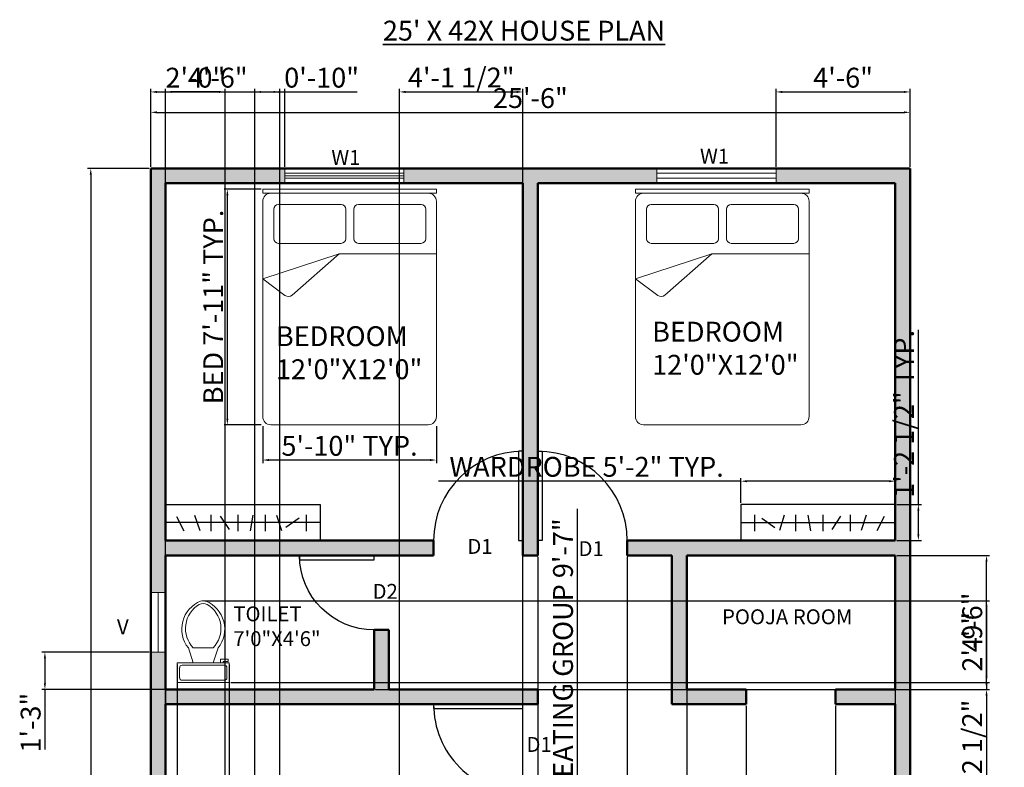
# Model space of a CAD drawing. Units: inches. Extents: x 3655 to 4051, y 2160 to 2854.
# Tile 3 of 3: x 3655 to 4051, y 2552 to 2854. Entities that reach past the tile are written whole.
import ezdxf

# ---------------------------------------------------------------- set-up
doc = ezdxf.new("R2010")
doc.units = ezdxf.units.IN
for name, color, linetype, lineweight in [('A-ANNO-DIMS', 2, 'Continuous', 18), ('A-ANNO-TEXT', 7, 'Continuous', 18), ('A-ANNO-TTLB', 7, 'Continuous', 35), ('A-AREA-IDEN', 7, 'Continuous', 25), ('A-DOOR', 3, 'Continuous', 25), ('A-FLOR-CASE', 8, 'Continuous', 25), ('A-FLOR-FIXT', 9, 'Continuous', 18), ('A-FURN', 8, 'Continuous', 18), ('A-GLAZ', 4, 'Continuous', 18), ('A-WALL', 7, 'Continuous', 50)]:
    doc.layers.add(name, color=color, linetype=linetype, lineweight=lineweight)
doc.layers.add('A-WALL-PATT', color=244, linetype='Continuous', lineweight=13, true_color=0x991b1e)
doc.styles.get("Standard").update_dxf_attribs({"font": 'arial.ttf'})
doc.dimstyles.new('ISO-25', dxfattribs={"dimtxt": 8, "dimasz": 2.5, "dimexe": 1.25, "dimexo": 0.625, "dimtad": 1, "dimdec": 1, "dimlunit": 3, "dimtxsty": 'Standard', "dimcen": 2.5, "dimadec": 0, "dimazin": 0, "dimtfac": 1, "dimtdec": 1, "dimtmove": 0, "dimatfit": 3, "dimfxl": 1, "dimarcsym": 0})

# ---------------------------------------------------------------- blocks, each defined once
blk = doc.blocks.new('*U2')
for p, q in [((0, 0), (0, -6)), ((36, 0), (36, -6))]:
    blk.add_line(p, q)
blk.add_lwpolyline([(0, 0), (0, 36), (1.75, 36), (1.75, 0)], close=True)
blk.add_arc((0, 0), 36, 0, 90)
blk = doc.blocks.new('*U3')
for p, q in [((0, 0), (0, -6)), ((-36, 0), (-36, -6))]:
    blk.add_line(p, q)
blk.add_lwpolyline([(0, 0), (0, 36), (-1.75, 36), (-1.75, 0)], close=True)
blk.add_arc((0, 0), 36, 90, 180)
blk = doc.blocks.new('*U4')
for p, q in [((0, 0), (0, 6)), ((36, 0), (36, 6))]:
    blk.add_line(p, q)
blk.add_lwpolyline([(0, 0), (0, -36), (1.75, -36), (1.75, 0)], close=True)
blk.add_arc((0, 0), 36, 270, 0)
blk = doc.blocks.new('*U5')
for p, q in [((-30, 0), (-30, 6)), ((0, 0), (0, 6))]:
    blk.add_line(p, q)
blk.add_lwpolyline([(0, 0), (0, -30), (-1.75, -30), (-1.75, 0)], close=True)
blk.add_arc((0, 0), 30, 180, 270)
blk = doc.blocks.new('A$C164346CA')
for p, q in [((0, 2.035), (0, 2)), ((1.5, 2.035), (0, 2.035)), ((1.5, 2), (0, 2)), ((1.5, 2), (1.5, 2.035)), ((0, 1.93), (0, 0.07)), ((0.6731, 1.9024), (0.1319, 1.9024)), ((1.364, 1.9024), (0.8228, 1.9024)), ((1.5, 0.07), (1.5, 1.93)), ((0.0919, 1.8624), (0.0919, 1.6069)), ((0.7131, 1.6069), (0.7131, 1.8624)), ((0.7828, 1.8624), (0.7828, 1.6069)), ((1.404, 1.6069), (1.404, 1.8624)), ((0.1319, 1.5669), (0.6731, 1.5669)), ((0.8228, 1.5669), (1.364, 1.5669)), ((0.8395, 1.4761), (0, 1.4761)), ((0.8395, 1.4761), (1.2448, 1.12)), ((1.5, 1.2611), (0.8395, 1.4761)), ((1.3077, 1.1175), (1.5, 1.2611)), ((0.07, 0), (1.43, 0))]:
    blk.add_line(p, q)
for centre, radius, start, end in [((0.07, 1.93), 0.07, 90, 180), ((1.43, 1.93), 0.07, 0, 90), ((0.1319, 1.8624), 0.04, 90, 180), ((0.6731, 1.8624), 0.04, 0, 90), ((0.8228, 1.8624), 0.04, 90, 180), ((1.364, 1.8624), 0.04, 0, 90), ((0.1319, 1.6069), 0.04, 180, 270), ((0.6731, 1.6069), 0.04, 270, 0), ((0.8228, 1.6069), 0.04, 180, 270), ((1.364, 1.6069), 0.04, 270, 0), ((1.2778, 1.1575), 0.05, 228.69584, 306.75789), ((0.07, 0.07), 0.07, 180, 270), ((1.43, 0.07), 0.07, 270, 0)]:
    blk.add_arc(centre, radius, start, end)
blk = doc.blocks.new('*U11')
for p, q in [((9.5, -6), (9.5, -2)), ((-10, -8.5), (-8, -8.5)), ((-10, -9.5), (-10, -8.5)), ((-7, -9.5), (-10, -9.5)), ((-8, -8.5), (-8, -8)), ((-7, -8), (-7, -9.5)), ((-4, -8), (-6, -14)), ((4, -8), (6, -14)), ((4, -14), (-4, -14))]:
    blk.add_line(p, q)
blk.add_lwpolyline([(10.5, -8), (10.5, 0), (-10.5, 0), (-10.5, -8)], close=True)
for points in [[(-9.5, -2), (-9.5, -6)], [(8.5, -1), (-8.5, -1)], [(-8.5, -7), (8.5, -7)]]:
    blk.add_lwpolyline(points)
for centre, radius, start, end in [((-8.62, -1.88), 0.884, 81.8699, 188.1301), ((8.62, -1.88), 0.884, 351.8699, 98.1301), ((-8.62, -6.12), 0.884, 171.8699, 278.1301), ((8.62, -6.12), 0.884, 261.8699, 8.1301), ((3.52, -21.58), 12.17, 141.4691, 247.9714), ((4.2, -21.82), 11.33, 136.3677, 238.9468), ((-3.52, -21.58), 12.17, 292.0284, 38.5307), ((-4.2, -21.82), 11.33, 301.053, 43.6321), ((0, -27.88), 4, 245.7318, 294.2682), ((0, -29), 4, 254.8605, 285.1395)]:
    blk.add_arc(centre, radius, start, end)
blk = doc.blocks.new('*D12')
at = {"layer": 'A-ANNO-DIMS', "color": 0, "lineweight": -2, "transparency": 16777216}
for p, q in [((3707.41, 2794.32), (3707.41, 2817.52)), ((4013.41, 2794.32), (4013.41, 2817.52)), ((3709.91, 2816.27), (4010.91, 2816.27))]:
    blk.add_line(p, q, dxfattribs=at)
at = {"layer": 'A-ANNO-DIMS', "color": 0, "transparency": 16777216}
for points in [[(3709.91, 2816.68), (3709.91, 2815.85), (3707.41, 2816.27)], [(4010.91, 2816.68), (4010.91, 2815.85), (4013.41, 2816.27)]]:
    blk.add_solid(points, dxfattribs=at)
at = {"layer": 'Defpoints', "color": 0, "transparency": 16777216}
for p in [(4013.41, 2816.27), (3707.41, 2793.69), (4013.41, 2793.69)]:
    blk.add_point(p, dxfattribs=at)
at = {"layer": 'A-ANNO-DIMS', "color": 0, "transparency": 16777216, "insert": (3860.41, 2820.98), "char_height": 8, "attachment_point": 5}
blk.add_mtext('25\'-6"', dxfattribs=at)
blk = doc.blocks.new('*D13')
at = {"layer": 'A-ANNO-DIMS', "color": 0, "lineweight": -2, "transparency": 16777216}
for p, q in [((3706.78, 2793.69), (3682, 2793.69)), ((3683.25, 2791.19), (3683.25, 2270.19)), ((3706.78, 2267.69), (3682, 2267.69))]:
    blk.add_line(p, q, dxfattribs=at)
at = {"layer": 'A-ANNO-DIMS', "color": 0, "transparency": 16777216}
for points in [[(3682.83, 2791.19), (3683.66, 2791.19), (3683.25, 2793.69)], [(3682.83, 2270.19), (3683.66, 2270.19), (3683.25, 2267.69)]]:
    blk.add_solid(points, dxfattribs=at)
at = {"layer": 'Defpoints', "color": 0, "transparency": 16777216}
for p in [(3707.41, 2793.69), (3683.25, 2267.69), (3707.41, 2267.69)]:
    blk.add_point(p, dxfattribs=at)
at = {"layer": 'A-ANNO-DIMS', "color": 0, "transparency": 16777216, "insert": (3678.53, 2530.69), "char_height": 8, "attachment_point": 5, "rotation": 90}
blk.add_mtext('43\'-10"', dxfattribs=at)
blk = doc.blocks.new('WARDROBE-RAIL')
for p, q in [((0, 14.59), (62.23, 14.59)), ((62.23, 14.59), (62.23, 0)), ((4.45, 9.69), (7.39, 3.9)), ((11.7, 10.18), (13.76, 4.03)), ((18.16, 10.34), (18.16, 3.85)), ((21.98, 9.84), (25.56, 4.42)), ((29.16, 10.34), (29.16, 3.85)), ((35.17, 10.28), (34.07, 3.88)), ((40.15, 10.34), (40.15, 3.85)), ((44.73, 10.2), (46.68, 4.01)), ((53.78, 8.99), (48.5, 5.2)), ((56.64, 10.34), (56.64, 3.85)), ((62.23, 7.29), (0, 7.29))]:
    blk.add_line(p, q)
blk = doc.blocks.new('WIN-W1-48IN')
for p, q in [((0, 0), (0, 6)), ((48, 4), (0, 4)), ((48, 0), (48, 6)), ((48, 2), (0, 2))]:
    blk.add_line(p, q)
blk = doc.blocks.new('*D16')
at = {"layer": 'A-ANNO-DIMS', "color": 0, "lineweight": -2, "transparency": 16777216}
for p, q in [((3751.9, 2785.3), (3737.04, 2785.3)), ((3738.29, 2692.87), (3738.29, 2782.8)), ((3751.9, 2690.37), (3737.04, 2690.37))]:
    blk.add_line(p, q, dxfattribs=at)
at = {"layer": 'A-ANNO-DIMS', "color": 0, "transparency": 16777216}
for points in [[(3737.87, 2782.8), (3738.71, 2782.8), (3738.29, 2785.3)], [(3737.87, 2692.87), (3738.71, 2692.87), (3738.29, 2690.37)]]:
    blk.add_solid(points, dxfattribs=at)
at = {"layer": 'Defpoints', "color": 0, "transparency": 16777216}
for p in [(3738.29, 2785.3), (3752.53, 2785.3), (3752.53, 2690.37)]:
    blk.add_point(p, dxfattribs=at)
at = {"layer": 'A-ANNO-DIMS', "color": 0, "transparency": 16777216, "insert": (3733.64, 2737.84), "char_height": 8, "attachment_point": 5, "rotation": 90}
blk.add_mtext('BED 7\'-11" TYP.', dxfattribs=at)
blk = doc.blocks.new('*D17')
at = {"layer": 'A-ANNO-DIMS', "color": 0, "lineweight": -2, "transparency": 16777216}
for p, q in [((3752.53, 2689.74), (3752.53, 2674.88)), ((3822.51, 2689.74), (3822.51, 2674.88)), ((3820.01, 2676.13), (3755.03, 2676.13))]:
    blk.add_line(p, q, dxfattribs=at)
at = {"layer": 'A-ANNO-DIMS', "color": 0, "transparency": 16777216}
for points in [[(3755.03, 2676.54), (3755.03, 2675.71), (3752.53, 2676.13)], [(3820.01, 2676.54), (3820.01, 2675.71), (3822.51, 2676.13)]]:
    blk.add_solid(points, dxfattribs=at)
at = {"layer": 'Defpoints', "color": 0, "transparency": 16777216}
for p in [(3752.53, 2690.37), (3822.51, 2690.37), (3752.53, 2676.13)]:
    blk.add_point(p, dxfattribs=at)
at = {"layer": 'A-ANNO-DIMS', "color": 0, "transparency": 16777216, "insert": (3787.52, 2680.84), "char_height": 8, "attachment_point": 5}
blk.add_mtext('5\'-10" TYP.', dxfattribs=at)
blk = doc.blocks.new('*D18')
at = {"layer": 'A-ANNO-DIMS', "color": 0, "lineweight": -2, "transparency": 16777216}
for p, q in [((3945.18, 2667.61), (3823.42, 2667.61)), ((3945.18, 2658.9), (3945.18, 2668.86)), ((4004.91, 2667.61), (3947.68, 2667.61)), ((4007.41, 2658.9), (4007.41, 2668.86))]:
    blk.add_line(p, q, dxfattribs=at)
at = {"layer": 'A-ANNO-DIMS', "color": 0, "transparency": 16777216}
for points in [[(3947.68, 2668.03), (3947.68, 2667.19), (3945.18, 2667.61)], [(4004.91, 2668.03), (4004.91, 2667.19), (4007.41, 2667.61)]]:
    blk.add_solid(points, dxfattribs=at)
at = {"layer": 'Defpoints', "color": 0, "transparency": 16777216}
for p in [(3945.18, 2667.61), (3945.18, 2658.28), (4007.41, 2658.28)]:
    blk.add_point(p, dxfattribs=at)
at = {"layer": 'A-ANNO-DIMS', "color": 0, "transparency": 16777216, "insert": (3883.05, 2672.37), "char_height": 8, "attachment_point": 5}
blk.add_mtext('WARDROBE 5\'-2" TYP.', dxfattribs=at)
blk = doc.blocks.new('*D19')
at = {"layer": 'A-ANNO-DIMS', "color": 0, "lineweight": -2, "transparency": 16777216}
for p, q in [((4016.74, 2658.28), (4016.74, 2728.68)), ((4008.03, 2658.28), (4017.99, 2658.28)), ((4016.74, 2646.19), (4016.74, 2655.78)), ((4008.03, 2643.69), (4017.99, 2643.69))]:
    blk.add_line(p, q, dxfattribs=at)
at = {"layer": 'A-ANNO-DIMS', "color": 0, "transparency": 16777216}
for points in [[(4016.33, 2655.78), (4017.16, 2655.78), (4016.74, 2658.28)], [(4016.33, 2646.19), (4017.16, 2646.19), (4016.74, 2643.69)]]:
    blk.add_solid(points, dxfattribs=at)
at = {"layer": 'Defpoints', "color": 0, "transparency": 16777216}
for p in [(4007.41, 2658.28), (4016.74, 2658.28), (4007.41, 2643.69)]:
    blk.add_point(p, dxfattribs=at)
at = {"layer": 'A-ANNO-DIMS', "color": 0, "transparency": 16777216, "insert": (4011.98, 2694.73), "char_height": 8, "attachment_point": 5, "rotation": 90}
blk.add_mtext('1\'-2 1/2" TYP.', dxfattribs=at)
blk = doc.blocks.new('*D22')
at = {"layer": 'A-ANNO-DIMS', "color": 0, "lineweight": -2, "transparency": 16777216}
for p, q in [((3879.35, 2535.27), (3879.35, 2656.5)), ((3895.99, 2535.27), (3878.1, 2535.27)), ((3879.35, 2422.65), (3879.35, 2532.77)), ((3895.99, 2420.15), (3878.1, 2420.15))]:
    blk.add_line(p, q, dxfattribs=at)
at = {"layer": 'A-ANNO-DIMS', "color": 0, "transparency": 16777216}
for points in [[(3878.93, 2532.77), (3879.76, 2532.77), (3879.35, 2535.27)], [(3878.93, 2422.65), (3879.76, 2422.65), (3879.35, 2420.15)]]:
    blk.add_solid(points, dxfattribs=at)
at = {"layer": 'Defpoints', "color": 0, "transparency": 16777216}
for p in [(3879.35, 2535.27), (3896.61, 2535.27), (3896.61, 2420.15)]:
    blk.add_point(p, dxfattribs=at)
at = {"layer": 'A-ANNO-DIMS', "color": 0, "transparency": 16777216, "insert": (3874.58, 2597.13), "char_height": 8, "attachment_point": 5, "rotation": 90}
blk.add_mtext('SEATING GROUP 9\'-7"', dxfattribs=at)
blk = doc.blocks.new('*D26')
at = {"layer": 'A-ANNO-DIMS', "color": 0, "lineweight": -2, "transparency": 16777216}
for p, q in [((3923.41, 2637.07), (3923.41, 2216.63)), ((4007.41, 2637.07), (4007.41, 2216.63)), ((3925.91, 2217.88), (4004.91, 2217.88))]:
    blk.add_line(p, q, dxfattribs=at)
at = {"layer": 'A-ANNO-DIMS', "color": 0, "transparency": 16777216}
for points in [[(3925.91, 2218.3), (3925.91, 2217.47), (3923.41, 2217.88)], [(4004.91, 2218.3), (4004.91, 2217.47), (4007.41, 2217.88)]]:
    blk.add_solid(points, dxfattribs=at)
at = {"layer": 'Defpoints', "color": 0, "transparency": 16777216}
for p in [(3923.41, 2637.69), (4007.41, 2637.69), (4007.41, 2217.88)]:
    blk.add_point(p, dxfattribs=at)
at = {"layer": 'A-ANNO-DIMS', "color": 0, "transparency": 16777216, "insert": (3965.41, 2222.59), "char_height": 8, "attachment_point": 5}
blk.add_mtext('7\'-0"', dxfattribs=at)
blk = doc.blocks.new('*D27')
at = {"layer": 'A-ANNO-DIMS', "color": 0, "lineweight": -2, "transparency": 16777216}
for p, q in [((4008.03, 2637.69), (4045.46, 2637.69)), ((4044.21, 2586.19), (4044.21, 2635.19)), ((4008.03, 2583.69), (4045.46, 2583.69))]:
    blk.add_line(p, q, dxfattribs=at)
at = {"layer": 'A-ANNO-DIMS', "color": 0, "transparency": 16777216}
for points in [[(4043.79, 2635.19), (4044.63, 2635.19), (4044.21, 2637.69)], [(4043.79, 2586.19), (4044.63, 2586.19), (4044.21, 2583.69)]]:
    blk.add_solid(points, dxfattribs=at)
at = {"layer": 'Defpoints', "color": 0, "transparency": 16777216}
for p in [(4007.41, 2637.69), (4044.21, 2637.69), (4007.41, 2583.69)]:
    blk.add_point(p, dxfattribs=at)
at = {"layer": 'A-ANNO-DIMS', "color": 0, "transparency": 16777216, "insert": (4039.5, 2610.69), "char_height": 8, "attachment_point": 5, "rotation": 90}
blk.add_mtext('4\'-6"', dxfattribs=at)
blk = doc.blocks.new('*D28')
at = {"layer": 'A-ANNO-DIMS', "color": 0, "lineweight": -2, "transparency": 16777216}
for p, q in [((3947.41, 2577.07), (3947.41, 2216.63)), ((3983.41, 2577.07), (3983.41, 2216.63)), ((3949.91, 2217.88), (3980.91, 2217.88))]:
    blk.add_line(p, q, dxfattribs=at)
at = {"layer": 'A-ANNO-DIMS', "color": 0, "transparency": 16777216}
for points in [[(3949.91, 2218.3), (3949.91, 2217.47), (3947.41, 2217.88)], [(3980.91, 2218.3), (3980.91, 2217.47), (3983.41, 2217.88)]]:
    blk.add_solid(points, dxfattribs=at)
at = {"layer": 'Defpoints', "color": 0, "transparency": 16777216}
for p in [(3947.41, 2577.69), (3983.41, 2577.69), (3983.41, 2217.88)]:
    blk.add_point(p, dxfattribs=at)
at = {"layer": 'A-ANNO-DIMS', "color": 0, "transparency": 16777216, "insert": (3965.41, 2222.59), "char_height": 8, "attachment_point": 5}
blk.add_mtext('3\'-0"', dxfattribs=at)
blk = doc.blocks.new('*D31')
at = {"layer": 'A-ANNO-DIMS', "color": 0, "lineweight": -2, "transparency": 16777216}
for p, q in [((3713.41, 2440.32), (3713.41, 2825.74)), ((3737.41, 2440.32), (3737.41, 2825.74)), ((3734.91, 2824.49), (3715.91, 2824.49))]:
    blk.add_line(p, q, dxfattribs=at)
at = {"layer": 'A-ANNO-DIMS', "color": 0, "transparency": 16777216}
for points in [[(3715.91, 2824.91), (3715.91, 2824.07), (3713.41, 2824.49)], [(3734.91, 2824.91), (3734.91, 2824.07), (3737.41, 2824.49)]]:
    blk.add_solid(points, dxfattribs=at)
at = {"layer": 'Defpoints', "color": 0, "transparency": 16777216}
for p in [(3713.41, 2824.49), (3713.41, 2439.69), (3737.41, 2439.69)]:
    blk.add_point(p, dxfattribs=at)
at = {"layer": 'A-ANNO-DIMS', "color": 0, "transparency": 16777216, "insert": (3725.41, 2829.2), "char_height": 8, "attachment_point": 5}
blk.add_mtext('2\'-0"', dxfattribs=at)
blk = doc.blocks.new('*D34')
at = {"layer": 'A-ANNO-DIMS', "color": 0, "lineweight": -2, "transparency": 16777216}
for p, q in [((3707.41, 2794.32), (3707.41, 2825.74)), ((3761.41, 2794.32), (3761.41, 2825.74)), ((3709.91, 2824.49), (3758.91, 2824.49))]:
    blk.add_line(p, q, dxfattribs=at)
at = {"layer": 'A-ANNO-DIMS', "color": 0, "transparency": 16777216}
for points in [[(3709.91, 2824.91), (3709.91, 2824.07), (3707.41, 2824.49)], [(3758.91, 2824.91), (3758.91, 2824.07), (3761.41, 2824.49)]]:
    blk.add_solid(points, dxfattribs=at)
at = {"layer": 'Defpoints', "color": 0, "transparency": 16777216}
for p in [(3761.41, 2824.49), (3707.41, 2793.69), (3761.41, 2793.69)]:
    blk.add_point(p, dxfattribs=at)
at = {"layer": 'A-ANNO-DIMS', "color": 0, "transparency": 16777216, "insert": (3734.41, 2829.2), "char_height": 8, "attachment_point": 5}
blk.add_mtext('4\'-6"', dxfattribs=at)
blk = doc.blocks.new('*D35')
at = {"layer": 'A-ANNO-DIMS', "color": 0, "lineweight": -2, "transparency": 16777216}
for p, q in [((3959.41, 2794.32), (3959.41, 2825.74)), ((4013.41, 2794.32), (4013.41, 2825.74)), ((3961.91, 2824.49), (4010.91, 2824.49))]:
    blk.add_line(p, q, dxfattribs=at)
at = {"layer": 'A-ANNO-DIMS', "color": 0, "transparency": 16777216}
for points in [[(3961.91, 2824.91), (3961.91, 2824.07), (3959.41, 2824.49)], [(4010.91, 2824.91), (4010.91, 2824.07), (4013.41, 2824.49)]]:
    blk.add_solid(points, dxfattribs=at)
at = {"layer": 'Defpoints', "color": 0, "transparency": 16777216}
for p in [(4013.41, 2824.49), (3959.41, 2793.69), (4013.41, 2793.69)]:
    blk.add_point(p, dxfattribs=at)
at = {"layer": 'A-ANNO-DIMS', "color": 0, "transparency": 16777216, "insert": (3986.41, 2829.2), "char_height": 8, "attachment_point": 5}
blk.add_mtext('4\'-6"', dxfattribs=at)
blk = doc.blocks.new('*D41')
at = {"layer": 'A-ANNO-DIMS', "color": 0, "lineweight": -2, "transparency": 16777216}
for p, q in [((3706.78, 2598.69), (3663.52, 2598.69)), ((3664.77, 2596.19), (3664.77, 2586.19)), ((3712.78, 2583.69), (3663.52, 2583.69)), ((3664.77, 2583.69), (3664.77, 2559.43))]:
    blk.add_line(p, q, dxfattribs=at)
at = {"layer": 'A-ANNO-DIMS', "color": 0, "transparency": 16777216}
for points in [[(3664.36, 2596.19), (3665.19, 2596.19), (3664.77, 2598.69)], [(3664.36, 2586.19), (3665.19, 2586.19), (3664.77, 2583.69)]]:
    blk.add_solid(points, dxfattribs=at)
at = {"layer": 'Defpoints', "color": 0, "transparency": 16777216}
for p in [(3707.41, 2598.69), (3664.77, 2583.69), (3713.41, 2583.69)]:
    blk.add_point(p, dxfattribs=at)
at = {"layer": 'A-ANNO-DIMS', "color": 0, "transparency": 16777216, "insert": (3660.06, 2570.31), "char_height": 8, "attachment_point": 5, "rotation": 90}
blk.add_mtext('1\'-3"', dxfattribs=at)
blk = doc.blocks.new('*D45')
at = {"layer": 'A-ANNO-DIMS', "color": 0, "lineweight": -2, "transparency": 16777216}
for p, q in [((3749.41, 2274.32), (3749.41, 2825.74)), ((3759.41, 2274.32), (3759.41, 2825.74)), ((3751.91, 2824.49), (3756.91, 2824.49)), ((3759.41, 2824.49), (3790.64, 2824.49))]:
    blk.add_line(p, q, dxfattribs=at)
at = {"layer": 'A-ANNO-DIMS', "color": 0, "transparency": 16777216}
for points in [[(3751.91, 2824.91), (3751.91, 2824.07), (3749.41, 2824.49)], [(3756.91, 2824.91), (3756.91, 2824.07), (3759.41, 2824.49)]]:
    blk.add_solid(points, dxfattribs=at)
at = {"layer": 'Defpoints', "color": 0, "transparency": 16777216}
for p in [(3759.41, 2824.49), (3749.41, 2273.69), (3759.41, 2273.69)]:
    blk.add_point(p, dxfattribs=at)
at = {"layer": 'A-ANNO-DIMS', "color": 0, "transparency": 16777216, "insert": (3776.28, 2829.2), "char_height": 8, "attachment_point": 5}
blk.add_mtext('0\'-10"', dxfattribs=at)
blk = doc.blocks.new('*D47')
at = {"layer": 'A-ANNO-DIMS', "color": 0, "lineweight": -2, "transparency": 16777216}
for p, q in [((3863.41, 2637.07), (3863.41, 2216.63)), ((3899.41, 2637.07), (3899.41, 2216.63)), ((3865.91, 2217.88), (3896.91, 2217.88))]:
    blk.add_line(p, q, dxfattribs=at)
at = {"layer": 'A-ANNO-DIMS', "color": 0, "transparency": 16777216}
for points in [[(3865.91, 2218.3), (3865.91, 2217.47), (3863.41, 2217.88)], [(3896.91, 2218.3), (3896.91, 2217.47), (3899.41, 2217.88)]]:
    blk.add_solid(points, dxfattribs=at)
at = {"layer": 'Defpoints', "color": 0, "transparency": 16777216}
for p in [(3863.41, 2637.69), (3899.41, 2637.69), (3899.41, 2217.88)]:
    blk.add_point(p, dxfattribs=at)
at = {"layer": 'A-ANNO-DIMS', "color": 0, "transparency": 16777216, "insert": (3881.41, 2222.59), "char_height": 8, "attachment_point": 5}
blk.add_mtext('3\'-0"', dxfattribs=at)
blk = doc.blocks.new('*D48')
at = {"layer": 'A-ANNO-DIMS', "color": 0, "lineweight": -2, "transparency": 16777216}
for p, q in [((3718.07, 2593.79), (3718.07, 2216.63)), ((3739.07, 2593.79), (3739.07, 2216.63)), ((3720.57, 2217.88), (3736.57, 2217.88)), ((3739.07, 2217.88), (3763.34, 2217.88))]:
    blk.add_line(p, q, dxfattribs=at)
at = {"layer": 'A-ANNO-DIMS', "color": 0, "transparency": 16777216}
for points in [[(3720.57, 2218.3), (3720.57, 2217.47), (3718.07, 2217.88)], [(3736.57, 2218.3), (3736.57, 2217.47), (3739.07, 2217.88)]]:
    blk.add_solid(points, dxfattribs=at)
at = {"layer": 'Defpoints', "color": 0, "transparency": 16777216}
for p in [(3718.07, 2594.42), (3739.07, 2594.42), (3739.07, 2217.88)]:
    blk.add_point(p, dxfattribs=at)
at = {"layer": 'A-ANNO-DIMS', "color": 0, "transparency": 16777216, "insert": (3752.46, 2222.59), "char_height": 8, "attachment_point": 5}
blk.add_mtext('1\'-9"', dxfattribs=at)
blk = doc.blocks.new('*D49')
at = {"layer": 'A-ANNO-DIMS', "color": 0, "lineweight": -2, "transparency": 16777216}
for p, q in [((3729.2, 2619.42), (4045.46, 2619.42)), ((4044.21, 2616.92), (4044.21, 2588.92)), ((3739.7, 2586.42), (4045.46, 2586.42))]:
    blk.add_line(p, q, dxfattribs=at)
at = {"layer": 'A-ANNO-DIMS', "color": 0, "transparency": 16777216}
for points in [[(4043.79, 2616.92), (4044.63, 2616.92), (4044.21, 2619.42)], [(4043.79, 2588.92), (4044.63, 2588.92), (4044.21, 2586.42)]]:
    blk.add_solid(points, dxfattribs=at)
at = {"layer": 'Defpoints', "color": 0, "transparency": 16777216}
for p in [(3728.57, 2619.42), (3739.07, 2586.42), (4044.21, 2586.42)]:
    blk.add_point(p, dxfattribs=at)
at = {"layer": 'A-ANNO-DIMS', "color": 0, "transparency": 16777216, "insert": (4039.5, 2602.92), "char_height": 8, "attachment_point": 5, "rotation": 90}
blk.add_mtext('2\'-9"', dxfattribs=at)
blk = doc.blocks.new('*D50')
at = {"layer": 'A-ANNO-DIMS', "color": 0, "lineweight": -2, "transparency": 16777216}
for p, q in [((3713.41, 2583.07), (3713.41, 2216.63)), ((3718.07, 2585.79), (3718.07, 2216.63)), ((3710.91, 2217.88), (3708.41, 2217.88)), ((3713.41, 2217.88), (3718.07, 2217.88)), ((3720.57, 2217.88), (3764.23, 2217.88))]:
    blk.add_line(p, q, dxfattribs=at)
at = {"layer": 'A-ANNO-DIMS', "color": 0, "transparency": 16777216}
for points in [[(3710.91, 2218.3), (3710.91, 2217.47), (3713.41, 2217.88)], [(3720.57, 2218.3), (3720.57, 2217.47), (3718.07, 2217.88)]]:
    blk.add_solid(points, dxfattribs=at)
at = {"layer": 'Defpoints', "color": 0, "transparency": 16777216}
for p in [(3713.41, 2583.69), (3718.07, 2586.42), (3718.07, 2217.88)]:
    blk.add_point(p, dxfattribs=at)
at = {"layer": 'A-ANNO-DIMS', "color": 0, "transparency": 16777216, "insert": (3743.65, 2222.64), "char_height": 8, "attachment_point": 5}
blk.add_mtext('0\'-4 1/2"', dxfattribs=at)
blk = doc.blocks.new('*D51')
at = {"layer": 'A-ANNO-DIMS', "color": 0, "lineweight": -2, "transparency": 16777216}
for p, q in [((4044.21, 2588.92), (4044.21, 2591.42)), ((3739.7, 2586.42), (4045.46, 2586.42)), ((3798.03, 2583.69), (4045.46, 2583.69)), ((4044.21, 2586.42), (4044.21, 2583.69)), ((4044.21, 2581.19), (4044.21, 2537.53))]:
    blk.add_line(p, q, dxfattribs=at)
at = {"layer": 'A-ANNO-DIMS', "color": 0, "transparency": 16777216}
for points in [[(4043.79, 2588.92), (4044.63, 2588.92), (4044.21, 2586.42)], [(4043.79, 2581.19), (4044.63, 2581.19), (4044.21, 2583.69)]]:
    blk.add_solid(points, dxfattribs=at)
at = {"layer": 'Defpoints', "color": 0, "transparency": 16777216}
for p in [(3739.07, 2586.42), (3797.41, 2583.69), (4044.21, 2583.69)]:
    blk.add_point(p, dxfattribs=at)
at = {"layer": 'A-ANNO-DIMS', "color": 0, "transparency": 16777216, "insert": (4039.45, 2558.11), "char_height": 8, "attachment_point": 5, "rotation": 90}
blk.add_mtext('0\'-2 1/2"', dxfattribs=at)
blk = doc.blocks.new('*D52')
at = {"layer": 'A-ANNO-DIMS', "color": 0, "lineweight": -2, "transparency": 16777216}
for p, q in [((3807.66, 2359.12), (3807.66, 2825.74)), ((3857.41, 2356.32), (3857.41, 2825.74)), ((3810.16, 2824.49), (3854.91, 2824.49))]:
    blk.add_line(p, q, dxfattribs=at)
at = {"layer": 'A-ANNO-DIMS', "color": 0, "transparency": 16777216}
for points in [[(3810.16, 2824.91), (3810.16, 2824.07), (3807.66, 2824.49)], [(3854.91, 2824.91), (3854.91, 2824.07), (3857.41, 2824.49)]]:
    blk.add_solid(points, dxfattribs=at)
at = {"layer": 'Defpoints', "color": 0, "transparency": 16777216}
for p in [(3857.41, 2824.49), (3807.66, 2358.5), (3857.41, 2355.69)]:
    blk.add_point(p, dxfattribs=at)
at = {"layer": 'A-ANNO-DIMS', "color": 0, "transparency": 16777216, "insert": (3832.54, 2829.25), "char_height": 8, "attachment_point": 5}
blk.add_mtext('4\'-1 1/2"', dxfattribs=at)

msp = doc.modelspace()

# ---------------------------------------------------------------- hatches: boundary and pattern name
at = {"layer": 'A-WALL-PATT'}
h = msp.add_hatch(color=256, dxfattribs=at)
h.dxf.hatch_style = 1
h.paths.add_polyline_path([(3713.41, 2787.69), (3761.41, 2787.69), (3761.41, 2793.69), (3707.41, 2793.69), (3707.41, 2622.69), (3713.41, 2622.69), (3713.41, 2637.69), (3821.41, 2637.69), (3821.41, 2643.69), (3713.41, 2643.69)])
h.paths.add_polyline_path([(3863.41, 2787.69), (3911.41, 2787.69), (3911.41, 2793.69), (3809.41, 2793.69), (3809.41, 2787.69), (3857.41, 2787.69), (3857.41, 2637.69), (3863.41, 2637.69)])
h.paths.add_polyline_path([(4013.41, 2793.69), (3959.41, 2793.69), (3959.41, 2787.69), (4007.41, 2787.69), (4007.41, 2643.69), (3899.41, 2643.69), (3899.41, 2637.69), (3917.41, 2637.69), (3917.41, 2577.69), (3947.41, 2577.69), (3947.41, 2583.69), (3923.41, 2583.69), (3923.41, 2637.69), (4007.41, 2637.69), (4007.41, 2583.69), (3983.41, 2583.69), (3983.41, 2577.69), (4007.41, 2577.69), (4007.41, 2500.75), (4013.41, 2500.75)])
h.paths.add_polyline_path([(3863.41, 2583.69), (3803.41, 2583.69), (3803.41, 2607.69), (3797.41, 2607.69), (3797.41, 2583.69), (3713.41, 2583.69), (3713.41, 2598.69), (3707.41, 2598.69), (3707.41, 2535.69), (3713.41, 2535.69), (3713.41, 2577.69), (3863.41, 2577.69)])
h.paths.add_polyline_path([(3863.41, 2541.69), (3857.41, 2541.69), (3857.41, 2445.69), (3713.41, 2445.69), (3713.41, 2487.69), (3707.41, 2487.69), (3707.41, 2421.69), (3713.41, 2421.69), (3713.41, 2439.69), (3857.41, 2439.69), (3857.41, 2415.69), (3863.41, 2415.69)])
h.paths.add_polyline_path([(3863.41, 2379.69), (3857.41, 2379.69), (3857.41, 2355.69), (3713.41, 2355.69), (3713.41, 2373.69), (3707.41, 2373.69), (3707.41, 2267.69), (3907.77, 2267.69), (3907.77, 2273.69), (3713.41, 2273.69), (3713.41, 2349.69), (3863.41, 2349.69)])
h.paths.add_polyline_path([(3951.59, 2273.69), (3943.77, 2273.69), (3943.77, 2267.69), (3951.59, 2267.69)])
h.paths.add_polyline_path([(4013.41, 2452.75), (4007.41, 2452.75), (4007.41, 2273.69), (3999.59, 2273.69), (3999.59, 2267.69), (4013.41, 2267.69)])

# ---------------------------------------------------------------- linework, layer by layer
at = {"layer": 'A-GLAZ'}
for p, q in [((3761.41, 2787.69), (3761.41, 2793.69)), ((3809.41, 2787.69), (3809.41, 2793.69)), ((3809.41, 2791.69), (3761.41, 2791.69)), ((3809.41, 2790.69), (3761.41, 2790.69)), ((3809.41, 2789.69), (3761.41, 2789.69)), ((3713.41, 2622.69), (3707.41, 2622.69)), ((3710.41, 2622.69), (3710.41, 2598.69)), ((3713.41, 2598.69), (3707.41, 2598.69))]:
    msp.add_line(p, q, dxfattribs=at)
at = {"layer": 'A-WALL'}
for p, q in [((3707.41, 2793.69), (3707.41, 2267.69)), ((3707.41, 2793.69), (4013.41, 2793.69)), ((4013.41, 2793.69), (4013.41, 2267.69)), ((3713.41, 2787.69), (3713.41, 2643.69)), ((3713.41, 2787.69), (3857.41, 2787.69)), ((3857.41, 2787.69), (3857.41, 2637.69)), ((3863.41, 2787.69), (3863.41, 2637.69)), ((3863.41, 2787.69), (4007.41, 2787.69)), ((4007.41, 2787.69), (4007.41, 2643.69)), ((3713.41, 2643.69), (3821.41, 2643.69)), ((3821.41, 2643.69), (3821.41, 2637.69)), ((3899.41, 2643.69), (4007.41, 2643.69)), ((3899.41, 2643.69), (3899.41, 2637.69)), ((3713.41, 2637.69), (3821.41, 2637.69)), ((3713.41, 2637.69), (3713.41, 2583.69)), ((3863.41, 2637.69), (3857.41, 2637.69)), ((3899.41, 2637.69), (3917.41, 2637.69)), ((3917.41, 2637.69), (3917.41, 2577.69)), ((3923.41, 2637.69), (3923.41, 2583.69)), ((3923.41, 2637.69), (4007.41, 2637.69)), ((4007.41, 2637.69), (4007.41, 2583.69)), ((3797.41, 2607.69), (3797.41, 2583.69)), ((3797.41, 2607.69), (3803.41, 2607.69)), ((3803.41, 2607.69), (3803.41, 2583.69)), ((3713.41, 2583.69), (3797.41, 2583.69)), ((3803.41, 2583.69), (3863.41, 2583.69)), ((3863.41, 2583.69), (3863.41, 2577.69)), ((3923.41, 2583.69), (3947.41, 2583.69)), ((3947.41, 2583.69), (3947.41, 2577.69)), ((3983.41, 2583.69), (3983.41, 2577.69)), ((3983.41, 2583.69), (4007.41, 2583.69)), ((3713.41, 2577.69), (3863.41, 2577.69)), ((3713.41, 2577.69), (3713.41, 2445.69)), ((3917.41, 2577.69), (3947.41, 2577.69)), ((3983.41, 2577.69), (4007.41, 2577.69)), ((4007.41, 2577.69), (4007.41, 2273.69))]:
    msp.add_line(p, q, dxfattribs=at)

# ---------------------------------------------------------------- block references
at = {"layer": 'A-DOOR'}
for name, p in [('*U3', (3857.41, 2643.69)), ('*U2', (3863.41, 2643.69))]:
    msp.add_blockref(name, p, dxfattribs=at)
at = {"layer": 'A-DOOR', "xscale": -1, "rotation": 270}
msp.add_blockref('*U5', (3797.41, 2637.69), dxfattribs=at)
at = {"layer": 'A-DOOR', "rotation": 270}
msp.add_blockref('*U4', (3857.41, 2577.69), dxfattribs=at)
at = {"layer": 'A-FLOR-CASE'}
msp.add_blockref('WARDROBE-RAIL', (3713.41, 2643.69), dxfattribs=at)
at = {"layer": 'A-FLOR-CASE', "extrusion": (0, 0, -1), "zscale": -1}
msp.add_blockref('WARDROBE-RAIL', (-4007.41, 2643.69), dxfattribs=at)
at = {"layer": 'A-FLOR-FIXT', "rotation": 180}
msp.add_blockref('*U11', (3728.57, 2586.42), dxfattribs=at)
at = {"layer": 'A-FURN', "xscale": -46.65071231409348, "yscale": 46.65071231409348, "zscale": 46.65071231409348}
for p in [(3822.51, 2690.37), (3972.71, 2690.37)]:
    msp.add_blockref('A$C164346CA', p, dxfattribs=at)
at = {"layer": 'A-GLAZ'}
msp.add_blockref('WIN-W1-48IN', (3911.41, 2787.69), dxfattribs=at)

# ---------------------------------------------------------------- texts
at = {"layer": 'A-ANNO-TEXT', "char_height": 6, "attachment_point": 1}
for s, insert in [('W1', (3928.74, 2801.59)), ('W1', (3780.19, 2801.09)), ('D1', (3835.02, 2644.33)), ('D1', (3879.82, 2643.43)), ('D2', (3796.82, 2626.21)), ('V', (3693.81, 2611.89)), ('D1', (3858.84, 2564.53))]:
    msp.add_mtext_dynamic_manual_height_columns(s, width=13.8821, gutter_width=12.5, heights=[0], dxfattribs=dict(at, insert=insert))
at = {"layer": 'A-ANNO-TTLB', "insert": (3800.96, 2853.19), "char_height": 8, "attachment_point": 1}
msp.add_mtext_dynamic_manual_height_columns("{\\L25' X 42X HOUSE PLAN}", width=259.49, gutter_width=12.5, heights=[0], dxfattribs=at)
at = {"layer": 'A-AREA-IDEN', "attachment_point": 1}
for s, insert, char_height in [('BEDROOM\\P12\'0"X12\'0"', (3757.86, 2730.06), 8), ('BEDROOM\\P12\'0"X12\'0"', (3909.47, 2731.87), 8), ('TOILET\\P7\'0"X4\'6"', (3740.69, 2617.15), 6), ('POOJA ROOM', (3937.63, 2615.97), 6)]:
    msp.add_mtext_dynamic_manual_height_columns(s, width=84.0989, gutter_width=12.5, heights=[0], dxfattribs=dict(at, insert=insert, char_height=char_height))

# ---------------------------------------------------------------- dimensions: what is measured, and where the dimension line sits
at = {"layer": 'A-ANNO-DIMS'}
for base, p1, p2, override, picture, middle in [((3857.4098, 2824.4907), (3807.6627, 2358.4982), (3857.4098, 2355.6907), {"dimdec": 1, "dimlfac": 1, "dimrnd": 0, "dimzin": 1, "dimdsep": 46, "dimlunit": 4, "dimfrac": 2}, '*D52', (3832.5363, 2829.2521)), ((3761.41, 2824.49), (3707.41, 2793.69), (3761.41, 2793.69), {"dimdec": 1, "dimlfac": 1, "dimrnd": 0, "dimzin": 1, "dimdsep": 46, "dimlunit": 4, "dimfrac": 2}, '*D34', (3734.41, 2829.2)), ((3713.41, 2824.49), (3737.41, 2439.69), (3713.41, 2439.69), {"dimdec": 1, "dimlfac": 1, "dimrnd": 0, "dimzin": 1, "dimdsep": 46, "dimlunit": 4, "dimfrac": 2}, '*D31', (3725.41, 2829.2)), ((3759.41, 2824.49), (3749.41, 2273.69), (3759.41, 2273.69), {"dimdec": 1, "dimlfac": 1, "dimrnd": 0, "dimzin": 1, "dimdsep": 46, "dimlunit": 4, "dimfrac": 2}, '*D45', (3776.28, 2829.2)), ((4013.41, 2824.49), (3959.41, 2793.69), (4013.41, 2793.69), {"dimdec": 1, "dimlfac": 1, "dimrnd": 0, "dimzin": 1, "dimdsep": 46, "dimlunit": 4, "dimfrac": 2}, '*D35', (3986.41, 2829.2)), ((4013.41, 2816.27), (3707.41, 2793.69), (4013.41, 2793.69), {"dimclrd": 0, "dimclre": 0, "dimclrt": 0}, '*D12', (3860.41, 2820.98)), ((3899.41, 2217.88), (3863.41, 2637.69), (3899.41, 2637.69), {"dimdec": 1, "dimlfac": 1, "dimrnd": 0, "dimzin": 1, "dimdsep": 46, "dimlunit": 4, "dimfrac": 2}, '*D47', (3881.41, 2222.59)), ((4007.41, 2217.88), (3923.41, 2637.69), (4007.41, 2637.69), {"dimdec": 1, "dimlfac": 1, "dimrnd": 0, "dimzin": 1, "dimdsep": 46, "dimlunit": 4, "dimfrac": 2}, '*D26', (3965.41, 2222.59)), ((3739.07, 2217.88), (3718.07, 2594.42), (3739.07, 2594.42), {"dimdec": 1, "dimlfac": 1, "dimrnd": 0, "dimzin": 1, "dimdsep": 46, "dimlunit": 4, "dimfrac": 2}, '*D48', (3752.46, 2222.59)), ((3718.07, 2217.88), (3713.41, 2583.69), (3718.07, 2586.42), {"dimdec": 1, "dimlfac": 1, "dimrnd": 0, "dimzin": 1, "dimdsep": 46, "dimlunit": 4, "dimfrac": 2}, '*D50', (3743.65, 2222.64)), ((3983.41, 2217.88), (3947.41, 2577.69), (3983.41, 2577.69), {"dimdec": 1, "dimlfac": 1, "dimrnd": 0, "dimzin": 1, "dimdsep": 46, "dimlunit": 4, "dimfrac": 2}, '*D28', (3965.41, 2222.59))]:
    dim = msp.add_linear_dim(base=base, p1=p1, p2=p2, dimstyle='ISO-25', override=override, dxfattribs=at)
    dim.commit()
    dim.dimension.update_dxf_attribs({"geometry": picture, "text_midpoint": middle})
for base, p1, p2, override, picture, middle in [((3683.25, 2267.69), (3707.41, 2793.69), (3707.41, 2267.69), {"dimclrd": 0, "dimclre": 0, "dimclrt": 0}, '*D13', (3678.53, 2530.69)), ((4044.21, 2637.69), (4007.41, 2583.69), (4007.41, 2637.69), {"dimdec": 1, "dimlfac": 1, "dimrnd": 0, "dimzin": 1, "dimdsep": 46, "dimlunit": 4, "dimfrac": 2}, '*D27', (4039.5, 2610.69)), ((4044.21, 2586.42), (3728.57, 2619.42), (3739.07, 2586.42), {"dimdec": 1, "dimlfac": 1, "dimrnd": 0, "dimzin": 1, "dimdsep": 46, "dimlunit": 4, "dimfrac": 2}, '*D49', (4039.5, 2602.92)), ((3664.77, 2583.69), (3707.41, 2598.69), (3713.41, 2583.69), {"dimdec": 1, "dimlfac": 1, "dimrnd": 0, "dimzin": 1, "dimdsep": 46, "dimlunit": 4, "dimfrac": 2}, '*D41', (3660.06, 2570.31)), ((4044.21, 2583.69), (3739.07, 2586.42), (3797.41, 2583.69), {"dimdec": 1, "dimlfac": 1, "dimrnd": 0, "dimzin": 1, "dimdsep": 46, "dimlunit": 4, "dimfrac": 2}, '*D51', (4039.45, 2558.11))]:
    dim = msp.add_linear_dim(base=base, p1=p1, p2=p2, angle=90, dimstyle='ISO-25', override=override, dxfattribs=at)
    dim.commit()
    dim.dimension.update_dxf_attribs({"geometry": picture, "text_midpoint": middle})
for base, p1, p2, angle, text, picture, middle in [((3738.29, 2785.3), (3752.53, 2690.37), (3752.53, 2785.3), 90, 'BED <> TYP.', '*D16', (3733.64, 2737.84)), ((4016.74, 2658.28), (4007.41, 2643.69), (4007.41, 2658.28), 90, '<> TYP.', '*D19', (4011.98, 2694.73)), ((3752.53, 2676.13), (3822.51, 2690.37), (3752.53, 2690.37), 180, '<> TYP.', '*D17', (3787.52, 2680.84)), ((3945.18, 2667.61), (4007.41, 2658.28), (3945.18, 2658.28), 180, 'WARDROBE <> TYP.', '*D18', (3883.05, 2672.37)), ((3879.35, 2535.27), (3896.61, 2420.15), (3896.61, 2535.27), 90, 'SEATING GROUP <>', '*D22', (3874.58, 2597.13))]:
    dim = msp.add_linear_dim(base=base, p1=p1, p2=p2, angle=angle, text=text, dimstyle='ISO-25', override={"dimdec": 1, "dimlfac": 1, "dimrnd": 0, "dimzin": 1, "dimdsep": 46, "dimlunit": 4, "dimfrac": 2}, dxfattribs=at)
    dim.commit()
    dim.dimension.update_dxf_attribs({"geometry": picture, "text_midpoint": middle})

doc.saveas('drawing.dxf')
